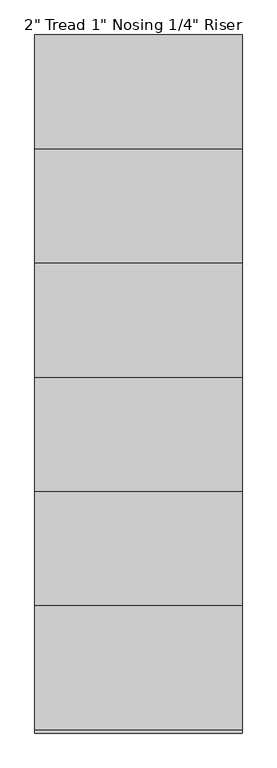
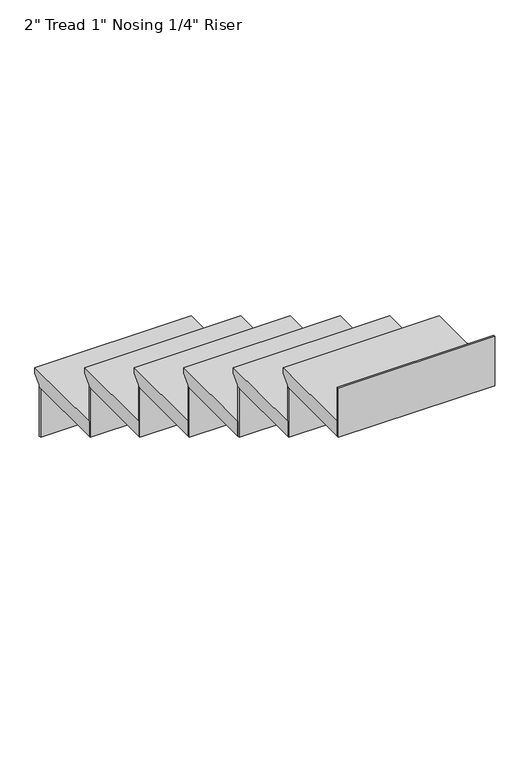
"""IFC4 building model written with IfcOpenShell, lengths in millimetres: stair flight geometry."""

from ifc_helpers import new_model, si_unit, frame, origin, place, context, project, spatial, polyline, outline, extrude, source, transform, mapped, element, save


def stair_flight_7fe2dcbd(model_context):
    return source(origin(), model_context, "Body", "SweptSolid", [
        extrude(outline(polyline([(-3107.7424149, 1354.6666667), (-2802.9424149, 1354.6666667), (-2802.9424149, 1335.6166667), (-2828.3424149, 1310.2166667), (-2828.3424149, 1303.8666667), (-3107.7424149, 1303.8666667), (-3107.7424149, 1354.6666667)])), frame((-620.2629117, 0.0, 0.0), z_axis=(1.0, 0.0, 0.0), x_axis=(0.0, 1.0, 0.0)), (0.0, 0.0, 1.0), 508.0),
        extrude(outline(polyline([(-620.2629117, -2834.6924149), (-620.2629117, -2828.3424149), (-112.2629117, -2828.3424149), (-112.2629117, -2834.6924149), (-620.2629117, -2834.6924149)])), frame((0.0, 0.0, 1134.5333333), z_axis=(0.0, 0.0, 1.0), x_axis=(1.0, 0.0, 0.0)), (0.0, 0.0, 1.0), 169.3333333),
        extrude(outline(polyline([(-620.2629117, -3114.0924149), (-620.2629117, -3107.7424149), (-112.2629117, -3107.7424149), (-112.2629117, -3114.0924149), (-620.2629117, -3114.0924149)])), frame((0.0, 0.0, 1303.8666667), z_axis=(0.0, 0.0, 1.0), x_axis=(1.0, 0.0, 0.0)), (0.0, 0.0, 1.0), 169.3333333),
        extrude(outline(polyline([(-3387.1424149, 1524.0), (-3082.3424149, 1524.0), (-3082.3424149, 1504.95), (-3107.7424149, 1479.55), (-3107.7424149, 1473.2), (-3387.1424149, 1473.2), (-3387.1424149, 1524.0)])), frame((-620.2629117, 0.0, 0.0), z_axis=(1.0, 0.0, 0.0), x_axis=(0.0, 1.0, 0.0)), (0.0, 0.0, 1.0), 508.0),
        extrude(outline(polyline([(-620.2629117, -3393.4924149), (-620.2629117, -3387.1424149), (-112.2629117, -3387.1424149), (-112.2629117, -3393.4924149), (-620.2629117, -3393.4924149)])), frame((0.0, 0.0, 1473.2), z_axis=(0.0, 0.0, 1.0), x_axis=(1.0, 0.0, 0.0)), (0.0, 0.0, 1.0), 169.3333333),
        extrude(outline(polyline([(-3666.5424149, 1693.3333333), (-3361.7424149, 1693.3333333), (-3361.7424149, 1674.2833333), (-3387.1424149, 1648.8833333), (-3387.1424149, 1642.5333333), (-3666.5424149, 1642.5333333), (-3666.5424149, 1693.3333333)])), frame((-620.2629117, 0.0, 0.0), z_axis=(1.0, 0.0, 0.0), x_axis=(0.0, 1.0, 0.0)), (0.0, 0.0, 1.0), 508.0),
        extrude(outline(polyline([(-620.2629117, -3672.8924149), (-620.2629117, -3666.5424149), (-112.2629117, -3666.5424149), (-112.2629117, -3672.8924149), (-620.2629117, -3672.8924149)])), frame((0.0, 0.0, 1642.5333333), z_axis=(0.0, 0.0, 1.0), x_axis=(1.0, 0.0, 0.0)), (0.0, 0.0, 1.0), 169.3333333),
        extrude(outline(polyline([(-3945.9424149, 1862.6666667), (-3641.1424149, 1862.6666667), (-3641.1424149, 1843.6166667), (-3666.5424149, 1818.2166667), (-3666.5424149, 1811.8666667), (-3945.9424149, 1811.8666667), (-3945.9424149, 1862.6666667)])), frame((-620.2629117, 0.0, 0.0), z_axis=(1.0, 0.0, 0.0), x_axis=(0.0, 1.0, 0.0)), (0.0, 0.0, 1.0), 508.0),
        extrude(outline(polyline([(-620.2629117, -3952.2924149), (-620.2629117, -3945.9424149), (-112.2629117, -3945.9424149), (-112.2629117, -3952.2924149), (-620.2629117, -3952.2924149)])), frame((0.0, 0.0, 1811.8666667), z_axis=(0.0, 0.0, 1.0), x_axis=(1.0, 0.0, 0.0)), (0.0, 0.0, 1.0), 169.3333333),
        extrude(outline(polyline([(-4225.3424149, 2032.0), (-3920.5424149, 2032.0), (-3920.5424149, 2012.95), (-3945.9424149, 1987.55), (-3945.9424149, 1981.2), (-4225.3424149, 1981.2), (-4225.3424149, 2032.0)])), frame((-620.2629117, 0.0, 0.0), z_axis=(1.0, 0.0, 0.0), x_axis=(0.0, 1.0, 0.0)), (0.0, 0.0, 1.0), 508.0),
        extrude(outline(polyline([(-620.2629117, -4231.6924149), (-620.2629117, -4225.3424149), (-112.2629117, -4225.3424149), (-112.2629117, -4231.6924149), (-620.2629117, -4231.6924149)])), frame((0.0, 0.0, 1981.2), z_axis=(0.0, 0.0, 1.0), x_axis=(1.0, 0.0, 0.0)), (0.0, 0.0, 1.0), 169.3333333),
        extrude(outline(polyline([(-620.2629117, -4511.0924149), (-620.2629117, -4504.7424149), (-112.2629117, -4504.7424149), (-112.2629117, -4511.0924149), (-620.2629117, -4511.0924149)])), frame((0.0, 0.0, 2150.5333333), z_axis=(0.0, 0.0, 1.0), x_axis=(1.0, 0.0, 0.0)), (0.0, 0.0, 1.0), 169.3333333),
        extrude(outline(polyline([(-4504.7424149, 2201.3333333), (-4199.9424149, 2201.3333333), (-4199.9424149, 2182.2833333), (-4225.3424149, 2156.8833333), (-4225.3424149, 2150.5333333), (-4504.7424149, 2150.5333333), (-4504.7424149, 2201.3333333)])), frame((-620.2629117, 0.0, 0.0), z_axis=(1.0, 0.0, 0.0), x_axis=(0.0, 1.0, 0.0)), (0.0, 0.0, 1.0), 508.0),
    ])


if __name__ == "__main__":
    model = new_model("IFC4")
    model_context = context("Model", 3, world=origin())
    ifc_project = project(units=[si_unit("LENGTHUNIT", "METRE", prefix="MILLI")], contexts=[model_context])
    site = spatial("IfcSite", under=ifc_project)
    building = spatial("IfcBuilding", under=site)
    placement = place(None, origin())
    stair_flight_shape = stair_flight_7fe2dcbd(model_context)
    element("IfcStairFlight", 1, ObjectType="2\" Tread 1\" Nosing 1/4\" Riser", at=placement, inside=building, context=model_context, shape_type="MappedRepresentation", body=[
        mapped(stair_flight_shape, transform((0.0, 0.0, 0.0), x_axis=(1.0, 0.0, 0.0), y_axis=(0.0, 1.0, 0.0), z_axis=(0.0, 0.0, 1.0))),
    ])
    save(model, "model.ifc")
